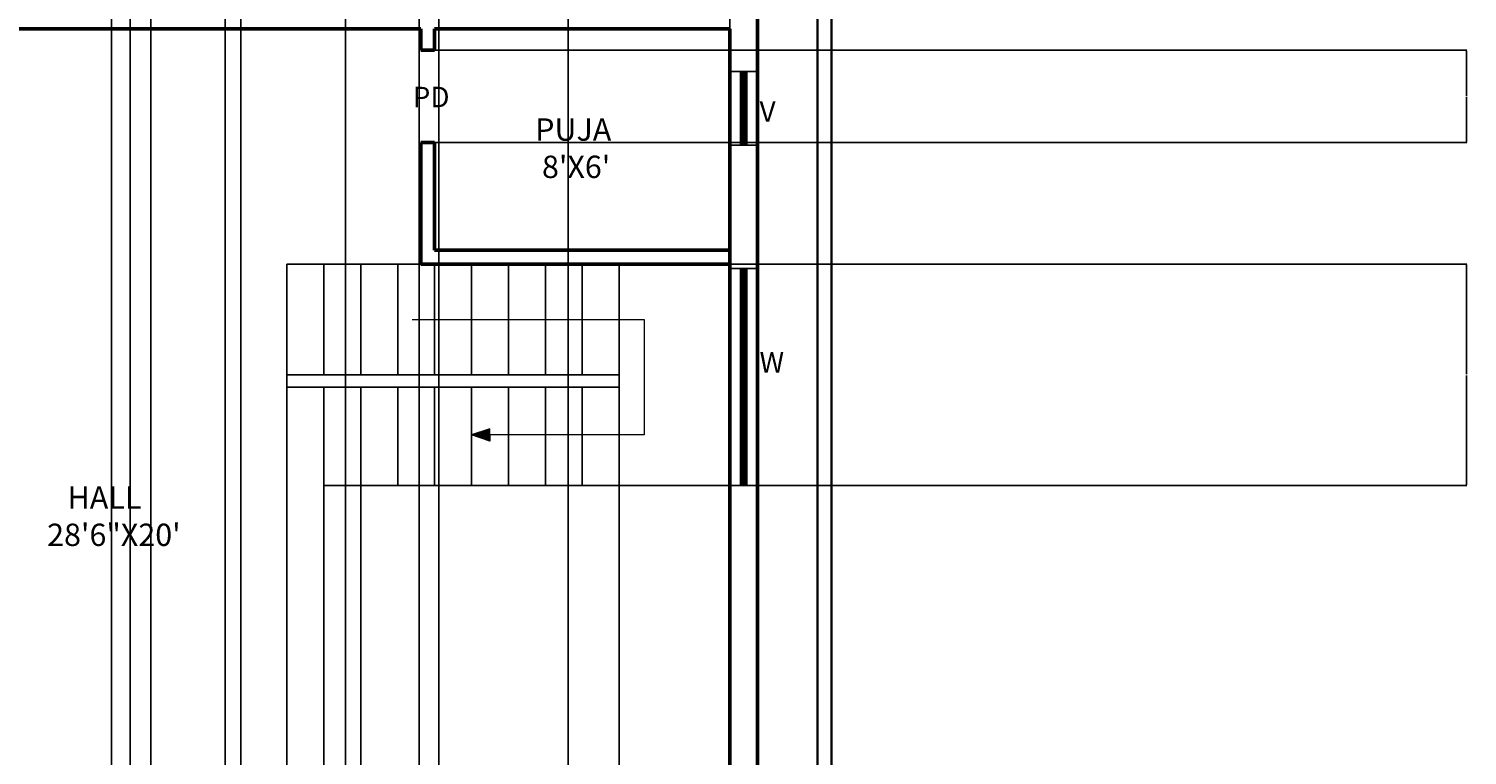
# Model space of a CAD drawing. Units: inches. Extents: x 338 to 1188, y -996 to 127.
# Tile 14 of 15: x 720 to 1188, y -385 to -149. Entities that reach past the tile are written whole.
import ezdxf

# ---------------------------------------------------------------- set-up
doc = ezdxf.new("R2010")
doc.units = ezdxf.units.IN
doc.header["$MEASUREMENT"] = 0
for name, color, linetype, lineweight in [('A-ANNO-DIMS', 5, 'Continuous', 18), ('A-ANNO-PATT', 7, 'Continuous', 13), ('A-ANNO-SYMB', 7, 'Continuous', 18), ('A-ANNO-TEXT', 7, 'Continuous', 18), ('A-AREA-IDEN', 8, 'Continuous', 18), ('A-FLOR-STRS', 7, 'Continuous', 25), ('A-GLAZ-PATT', 5, 'Continuous', 13), ('C-PROP', 1, 'Continuous', 35), ('wall', 1, 'Continuous', 50), ('win', 5, 'Continuous', 25)]:
    doc.layers.add(name, color=color, linetype=linetype, lineweight=lineweight)
doc.styles.get("Standard").update_dxf_attribs({"font": 'arial.ttf'})
doc.dimstyles.get("Standard").update_dxf_attribs({"dimtxt": 0.18, "dimasz": 0.18, "dimexe": 0.18, "dimexo": 0.0625, "dimgap": 0.09, "dimtad": 0, "dimtih": 1, "dimtoh": 1, "dimdec": 1, "dimzin": 0, "dimdsep": 46, "dimlunit": 4, "dimtxsty": 'Standard', "dimcen": 0.09, "dimadec": 0, "dimazin": 0, "dimtfac": 1, "dimtdec": 1, "dimtofl": 0, "dimtmove": 0, "dimatfit": 3, "dimfxl": 1, "dimtolj": 1, "dimtzin": 0, "dimarcsym": 0})

# ---------------------------------------------------------------- blocks, each defined once
blk = doc.blocks.new('*D26')
at = {"layer": 'A-ANNO-DIMS', "color": 0, "lineweight": -2, "transparency": 16777216}
for p, q in [((815.96, -297.8), (815.96, -968.86)), ((827.96, -297.8), (827.96, -968.86)), ((816.14, -968.68), (821.64, -968.68)), ((827.78, -968.68), (822.28, -968.68))]:
    blk.add_line(p, q, dxfattribs=at)
at = {"layer": 'A-ANNO-DIMS', "color": 0, "transparency": 16777216}
for points in [[(816.14, -968.65), (816.14, -968.71), (815.96, -968.68)], [(827.78, -968.65), (827.78, -968.71), (827.96, -968.68)]]:
    blk.add_solid(points, dxfattribs=at)
at = {"layer": 'Defpoints', "color": 0, "transparency": 16777216}
for p in [(815.96, -297.73), (827.96, -297.73), (827.96, -968.68)]:
    blk.add_point(p, dxfattribs=at)
at = {"layer": 'A-ANNO-DIMS', "color": 0, "transparency": 16777216, "insert": (821.96, -968.68), "char_height": 0.18, "attachment_point": 5}
blk.add_mtext('\\A1;1\'-0"', dxfattribs=at)
blk = doc.blocks.new('*D27')
at = {"layer": 'A-ANNO-DIMS', "color": 0, "lineweight": -2, "transparency": 16777216}
for p, q in [((911.96, -297.8), (911.96, -968.86)), ((947.96, -297.8), (947.96, -968.86)), ((912.14, -968.68), (929.63, -968.68)), ((947.78, -968.68), (930.29, -968.68))]:
    blk.add_line(p, q, dxfattribs=at)
at = {"layer": 'A-ANNO-DIMS', "color": 0, "transparency": 16777216}
for points in [[(912.14, -968.65), (912.14, -968.71), (911.96, -968.68)], [(947.78, -968.65), (947.78, -968.71), (947.96, -968.68)]]:
    blk.add_solid(points, dxfattribs=at)
at = {"layer": 'Defpoints', "color": 0, "transparency": 16777216}
for p in [(911.96, -297.73), (947.96, -297.73), (947.96, -968.68)]:
    blk.add_point(p, dxfattribs=at)
at = {"layer": 'A-ANNO-DIMS', "color": 0, "transparency": 16777216, "insert": (929.96, -968.68), "char_height": 0.18, "attachment_point": 5}
blk.add_mtext('\\A1;3\'-0"', dxfattribs=at)
blk = doc.blocks.new('*D28')
at = {"layer": 'A-ANNO-DIMS', "color": 0, "lineweight": -2, "transparency": 16777216}
for p, q in [((803.96, -265.8), (803.96, -968.86)), ((947.96, -297.8), (947.96, -968.86)), ((804.14, -968.68), (875.57, -968.68)), ((947.78, -968.68), (876.35, -968.68))]:
    blk.add_line(p, q, dxfattribs=at)
at = {"layer": 'A-ANNO-DIMS', "color": 0, "transparency": 16777216}
for points in [[(804.14, -968.65), (804.14, -968.71), (803.96, -968.68)], [(947.78, -968.65), (947.78, -968.71), (947.96, -968.68)]]:
    blk.add_solid(points, dxfattribs=at)
at = {"layer": 'Defpoints', "color": 0, "transparency": 16777216}
for p in [(803.96, -265.73), (947.96, -297.73), (947.96, -968.68)]:
    blk.add_point(p, dxfattribs=at)
at = {"layer": 'A-ANNO-DIMS', "color": 0, "transparency": 16777216, "insert": (875.96, -968.68), "char_height": 0.18, "attachment_point": 5}
blk.add_mtext('\\A1;12\'-0"', dxfattribs=at)
blk = doc.blocks.new('*D29')
at = {"layer": 'A-ANNO-DIMS', "color": 0, "lineweight": -2, "transparency": 16777216}
for p, q in [((948.03, -225.73), (1187.6, -225.73)), ((1187.42, -225.91), (1187.42, -261.55)), ((1187.42, -297.55), (1187.42, -261.91)), ((948.03, -297.73), (1187.6, -297.73))]:
    blk.add_line(p, q, dxfattribs=at)
at = {"layer": 'A-ANNO-DIMS', "color": 0, "transparency": 16777216}
for points in [[(1187.39, -225.91), (1187.45, -225.91), (1187.42, -225.73)], [(1187.39, -297.55), (1187.45, -297.55), (1187.42, -297.73)]]:
    blk.add_solid(points, dxfattribs=at)
at = {"layer": 'Defpoints', "color": 0, "transparency": 16777216}
for p in [(947.96, -225.73), (947.96, -297.73), (1187.42, -297.73)]:
    blk.add_point(p, dxfattribs=at)
at = {"layer": 'A-ANNO-DIMS', "color": 0, "transparency": 16777216, "insert": (1187.42, -261.73), "char_height": 0.18, "attachment_point": 5}
blk.add_mtext('\\A1;6\'-0"', dxfattribs=at)
blk = doc.blocks.new('*D37')
at = {"layer": 'A-ANNO-DIMS', "color": 0, "lineweight": -2, "transparency": 16777216}
for p, q in [((752.96, -393.67), (752.96, 67.25)), ((753.14, 67.07), (770.63, 67.07)), ((788.78, 67.07), (771.29, 67.07)), ((788.96, -393.67), (788.96, 67.25))]:
    blk.add_line(p, q, dxfattribs=at)
at = {"layer": 'A-ANNO-DIMS', "color": 0, "transparency": 16777216}
for points in [[(753.14, 67.1), (753.14, 67.04), (752.96, 67.07)], [(788.78, 67.1), (788.78, 67.04), (788.96, 67.07)]]:
    blk.add_solid(points, dxfattribs=at)
at = {"layer": 'Defpoints', "color": 0, "transparency": 16777216}
for p in [(788.96, 67.07), (752.96, -393.73), (788.96, -393.73)]:
    blk.add_point(p, dxfattribs=at)
at = {"layer": 'A-ANNO-DIMS', "color": 0, "transparency": 16777216, "insert": (770.96, 67.07), "char_height": 0.18, "attachment_point": 5}
blk.add_mtext('\\A1;3\'-0"', dxfattribs=at)
blk = doc.blocks.new('*D38')
at = {"layer": 'A-ANNO-DIMS', "color": 0, "lineweight": -2, "transparency": 16777216}
for p, q in [((822.96, -470.17), (822.96, 67.25)), ((823.14, 67.07), (834.63, 67.07)), ((846.78, 67.07), (835.29, 67.07)), ((846.96, -470.17), (846.96, 67.25))]:
    blk.add_line(p, q, dxfattribs=at)
at = {"layer": 'A-ANNO-DIMS', "color": 0, "transparency": 16777216}
for points in [[(823.14, 67.1), (823.14, 67.04), (822.96, 67.07)], [(846.78, 67.1), (846.78, 67.04), (846.96, 67.07)]]:
    blk.add_solid(points, dxfattribs=at)
at = {"layer": 'Defpoints', "color": 0, "transparency": 16777216}
for p in [(846.96, 67.07), (822.96, -470.23), (846.96, -470.23)]:
    blk.add_point(p, dxfattribs=at)
at = {"layer": 'A-ANNO-DIMS', "color": 0, "transparency": 16777216, "insert": (834.96, 67.07), "char_height": 0.18, "attachment_point": 5}
blk.add_mtext('\\A1;2\'-0"', dxfattribs=at)
blk = doc.blocks.new('*D39')
at = {"layer": 'A-ANNO-DIMS', "color": 0, "lineweight": -2, "transparency": 16777216}
for p, q in [((852.03, -156.23), (1187.6, -156.23)), ((1187.42, -156.41), (1187.42, -171.05)), ((1187.42, -186.05), (1187.42, -171.41)), ((852.03, -186.23), (1187.6, -186.23))]:
    blk.add_line(p, q, dxfattribs=at)
at = {"layer": 'A-ANNO-DIMS', "color": 0, "transparency": 16777216}
for points in [[(1187.39, -156.41), (1187.45, -156.41), (1187.42, -156.23)], [(1187.39, -186.05), (1187.45, -186.05), (1187.42, -186.23)]]:
    blk.add_solid(points, dxfattribs=at)
at = {"layer": 'Defpoints', "color": 0, "transparency": 16777216}
for p in [(851.96, -156.23), (851.96, -186.23), (1187.42, -186.23)]:
    blk.add_point(p, dxfattribs=at)
at = {"layer": 'A-ANNO-DIMS', "color": 0, "transparency": 16777216, "insert": (1187.42, -171.23), "char_height": 0.18, "attachment_point": 5}
blk.add_mtext('\\A1;2\'-6"', dxfattribs=at)
blk = doc.blocks.new('*D42')
at = {"layer": 'A-ANNO-DIMS', "color": 0, "lineweight": -2, "transparency": 16777216}
for p, q in [((746.96, -54.8), (746.96, -968.86)), ((783.89, -54.8), (783.89, -968.86)), ((747.14, -968.68), (765.1, -968.68)), ((783.71, -968.68), (765.76, -968.68))]:
    blk.add_line(p, q, dxfattribs=at)
at = {"layer": 'A-ANNO-DIMS', "color": 0, "transparency": 16777216}
for points in [[(747.14, -968.65), (747.14, -968.71), (746.96, -968.68)], [(783.71, -968.65), (783.71, -968.71), (783.89, -968.68)]]:
    blk.add_solid(points, dxfattribs=at)
at = {"layer": 'Defpoints', "color": 0, "transparency": 16777216}
for p in [(746.96, -54.73), (783.89, -54.73), (783.89, -968.68)]:
    blk.add_point(p, dxfattribs=at)
at = {"layer": 'A-ANNO-DIMS', "color": 0, "transparency": 16777216, "insert": (765.43, -968.68), "char_height": 0.18, "attachment_point": 5}
blk.add_mtext('\\A1;3\'-1"', dxfattribs=at)
blk = doc.blocks.new('*D43')
at = {"layer": 'A-ANNO-DIMS', "color": 0, "lineweight": -2, "transparency": 16777216}
for p, q in [((853.28, -53.93), (853.28, -968.86)), ((895.37, -53.93), (895.37, -968.86)), ((853.46, -968.68), (873.99, -968.68)), ((895.19, -968.68), (874.65, -968.68))]:
    blk.add_line(p, q, dxfattribs=at)
at = {"layer": 'A-ANNO-DIMS', "color": 0, "transparency": 16777216}
for points in [[(853.46, -968.65), (853.46, -968.71), (853.28, -968.68)], [(895.19, -968.65), (895.19, -968.71), (895.37, -968.68)]]:
    blk.add_solid(points, dxfattribs=at)
at = {"layer": 'Defpoints', "color": 0, "transparency": 16777216}
for p in [(853.28, -53.87), (895.37, -53.87), (895.37, -968.68)]:
    blk.add_point(p, dxfattribs=at)
at = {"layer": 'A-ANNO-DIMS', "color": 0, "transparency": 16777216, "insert": (874.32, -968.68), "char_height": 0.18, "attachment_point": 5}
blk.add_mtext('\\A1;3\'-6"', dxfattribs=at)
blk = doc.blocks.new('*D44')
at = {"layer": 'A-ANNO-DIMS', "color": 0, "lineweight": -2, "transparency": 16777216}
for p, q in [((895.37, -53.93), (895.37, -968.86)), ((947.96, -54.8), (947.96, -968.86)), ((895.55, -968.68), (921.12, -968.68)), ((947.78, -968.68), (922.21, -968.68))]:
    blk.add_line(p, q, dxfattribs=at)
at = {"layer": 'A-ANNO-DIMS', "color": 0, "transparency": 16777216}
for points in [[(895.55, -968.65), (895.55, -968.71), (895.37, -968.68)], [(947.78, -968.65), (947.78, -968.71), (947.96, -968.68)]]:
    blk.add_solid(points, dxfattribs=at)
at = {"layer": 'Defpoints', "color": 0, "transparency": 16777216}
for p in [(895.37, -53.87), (947.96, -54.73), (947.96, -968.68)]:
    blk.add_point(p, dxfattribs=at)
at = {"layer": 'A-ANNO-DIMS', "color": 0, "transparency": 16777216, "insert": (921.67, -968.68), "char_height": 0.18, "attachment_point": 5}
blk.add_mtext('\\A1;4\'-4 1/2"', dxfattribs=at)
blk = doc.blocks.new('*D47')
at = {"layer": 'A-ANNO-DIMS', "color": 0, "lineweight": -2, "transparency": 16777216}
for p, q in [((759.67, -755.17), (759.67, 67.25)), ((759.85, 67.07), (867.68, 67.07)), ((976.28, 67.07), (868.46, 67.07)), ((976.46, -755.17), (976.46, 67.25))]:
    blk.add_line(p, q, dxfattribs=at)
at = {"layer": 'A-ANNO-DIMS', "color": 0, "transparency": 16777216}
for points in [[(759.85, 67.1), (759.85, 67.04), (759.67, 67.07)], [(976.28, 67.1), (976.28, 67.04), (976.46, 67.07)]]:
    blk.add_solid(points, dxfattribs=at)
at = {"layer": 'Defpoints', "color": 0, "transparency": 16777216}
for p in [(976.46, 67.07), (759.67, -755.23), (976.46, -755.23)]:
    blk.add_point(p, dxfattribs=at)
at = {"layer": 'A-ANNO-DIMS', "color": 0, "transparency": 16777216, "insert": (868.07, 67.07), "char_height": 0.18, "attachment_point": 5}
blk.add_mtext('\\A1;18\'-1"', dxfattribs=at)

msp = doc.modelspace()

# ---------------------------------------------------------------- hatches: boundary and pattern name
at = {"layer": 'A-ANNO-PATT'}
h = msp.add_hatch(dxfattribs=at)
h.set_pattern_fill('ANSI31', color=256)
h.paths.add_polyline_path([(869.89, -281.26), (869.89, -279.26), (863.96, -281.26), (869.89, -283.26)])
at = {"layer": 'A-GLAZ-PATT'}
h = msp.add_hatch(dxfattribs=at)
h.set_pattern_fill('ANSI31', color=256)
h.paths.add_polyline_path([(953.46, -98.96), (951.46, -98.96), (951.46, -134.96), (953.46, -134.96)])
h.paths.add_polyline_path([(953.46, -163.12), (951.46, -163.12), (951.46, -187.12), (953.46, -187.12)])
h.paths.add_polyline_path([(953.46, -227.22), (951.46, -227.22), (951.46, -297.73), (953.46, -297.73)])

# ---------------------------------------------------------------- linework, layer by layer
at = {"layer": 'A-ANNO-SYMB'}
for p, q in [((844.64, -243.73), (920.14, -243.73)), ((920.14, -243.73), (920.14, -281.26)), ((869.89, -279.26), (863.96, -281.26)), ((869.89, -281.26), (869.89, -279.26)), ((869.89, -283.26), (863.96, -281.26)), ((920.14, -281.26), (869.89, -281.26)), ((869.89, -281.26), (869.89, -283.26))]:
    msp.add_line(p, q, dxfattribs=at)
at = {"layer": 'A-FLOR-STRS'}
for p, q in [((847.46, -225.73), (803.96, -225.73)), ((803.96, -225.73), (803.96, -265.73)), ((815.96, -225.73), (815.96, -261.73)), ((827.96, -225.73), (827.96, -261.73)), ((839.96, -225.73), (839.96, -261.73)), ((851.96, -225.73), (851.96, -261.73)), ((863.96, -225.73), (863.96, -261.73)), ((875.96, -225.73), (875.96, -261.73)), ((887.96, -225.73), (887.96, -261.73)), ((899.96, -225.73), (899.96, -261.73)), ((911.96, -225.73), (911.96, -297.73)), ((911.96, -261.73), (803.96, -261.73)), ((911.96, -265.73), (803.96, -265.73)), ((815.96, -265.73), (815.96, -297.73)), ((827.96, -265.73), (827.96, -297.73)), ((839.96, -265.73), (839.96, -297.73)), ((851.96, -265.73), (851.96, -297.73)), ((863.96, -265.73), (863.96, -297.73)), ((875.96, -265.73), (875.96, -297.73)), ((887.96, -265.73), (887.96, -297.73)), ((899.96, -265.73), (899.96, -297.73)), ((947.96, -297.73), (815.96, -297.73))]:
    msp.add_line(p, q, dxfattribs=at)
at = {"layer": 'C-PROP'}
for p, q in [((980.96, 8.27), (980.96, -807.73)), ((976.46, 3.77), (976.46, -803.23))]:
    msp.add_line(p, q, dxfattribs=at)
at = {"layer": 'wall'}
for p, q in [((956.96, -15.73), (956.96, -615.73)), ((847.46, -149.23), (701.96, -149.23)), ((847.46, -149.23), (847.46, -156.23)), ((947.96, -149.23), (851.96, -149.23)), ((851.96, -149.23), (851.96, -156.23)), ((947.96, -149.23), (947.96, -393.73)), ((851.96, -156.23), (847.46, -156.23)), ((851.96, -186.23), (847.46, -186.23)), ((847.46, -186.23), (847.46, -225.73)), ((851.96, -186.23), (851.96, -221.23)), ((947.96, -221.23), (851.96, -221.23)), ((947.96, -225.73), (847.46, -225.73))]:
    msp.add_line(p, q, dxfattribs=at)
at = {"layer": 'win'}
for p, q in [((947.96, -163.12), (956.96, -163.12)), ((951.46, -163.12), (951.46, -187.12)), ((953.46, -163.12), (953.46, -187.12)), ((947.96, -187.12), (956.96, -187.12)), ((947.96, -227.22), (956.96, -227.22)), ((951.46, -227.22), (951.46, -297.73)), ((953.46, -227.22), (953.46, -297.73)), ((947.96, -297.73), (956.96, -297.73))]:
    msp.add_line(p, q, dxfattribs=at)

# ---------------------------------------------------------------- texts
at = {"layer": 'A-ANNO-TEXT'}
for s, height, p in [('PD', 6.652, (844.83, -174.74)), ('V', 6.65, (957.61, -179.47)), ('W', 6.65, (957.61, -260.99))]:
    msp.add_text(s, height=height, dxfattribs=at).set_placement(p)
at = {"layer": 'A-AREA-IDEN', "char_height": 7.27, "attachment_point": 1}
for s, width, insert in [("    PUJA\\P     8'X6'", 40.9908, (875.76, -178.37)), ('    HALL\\P 28\'6"X20\'', 49.0638, (723.75, -298))]:
    msp.add_mtext_dynamic_manual_height_columns(s, width=width, gutter_width=1, heights=[0], dxfattribs=dict(at, insert=insert))

# ---------------------------------------------------------------- dimensions: what is measured, and where the dimension line sits
at = {"layer": 'A-ANNO-DIMS'}
for base, p1, p2, picture, middle in [((788.96, 67.07), (752.96, -393.73), (788.96, -393.73), '*D37', (770.96, 67.07)), ((976.46, 67.07), (759.67, -755.23), (976.46, -755.23), '*D47', (868.07, 67.07)), ((846.96, 67.07), (822.96, -470.23), (846.96, -470.23), '*D38', (834.96, 67.07)), ((783.89, -968.68), (746.96, -54.73), (783.89, -54.73), '*D42', (765.43, -968.68)), ((895.37, -968.68), (853.28, -53.87), (895.37, -53.87), '*D43', (874.32, -968.68)), ((947.96, -968.68), (895.37, -53.87), (947.96, -54.73), '*D44', (921.67, -968.68)), ((947.96, -968.68), (803.96, -265.73), (947.96, -297.73), '*D28', (875.96, -968.68)), ((827.96, -968.68), (815.96, -297.73), (827.96, -297.73), '*D26', (821.96, -968.68)), ((947.96, -968.68), (911.96, -297.73), (947.96, -297.73), '*D27', (929.96, -968.68))]:
    dim = msp.add_linear_dim(base=base, p1=p1, p2=p2, dimstyle='Standard', override={"dimdec": 1, "dimlfac": 1, "dimrnd": 0, "dimzin": 1, "dimdsep": 46, "dimlunit": 4, "dimfrac": 2}, dxfattribs=at)
    dim.commit()
    dim.dimension.update_dxf_attribs({"geometry": picture, "text_midpoint": middle})
for base, p1, p2, picture, middle in [((1187.42, -186.23), (851.96, -156.23), (851.96, -186.23), '*D39', (1187.42, -171.23)), ((1187.42, -297.73), (947.96, -225.73), (947.96, -297.73), '*D29', (1187.42, -261.73))]:
    dim = msp.add_linear_dim(base=base, p1=p1, p2=p2, angle=90, dimstyle='Standard', override={"dimdec": 1, "dimlfac": 1, "dimrnd": 0, "dimzin": 1, "dimdsep": 46, "dimlunit": 4, "dimfrac": 2}, dxfattribs=at)
    dim.commit()
    dim.dimension.update_dxf_attribs({"geometry": picture, "text_midpoint": middle})

doc.saveas('drawing.dxf')
